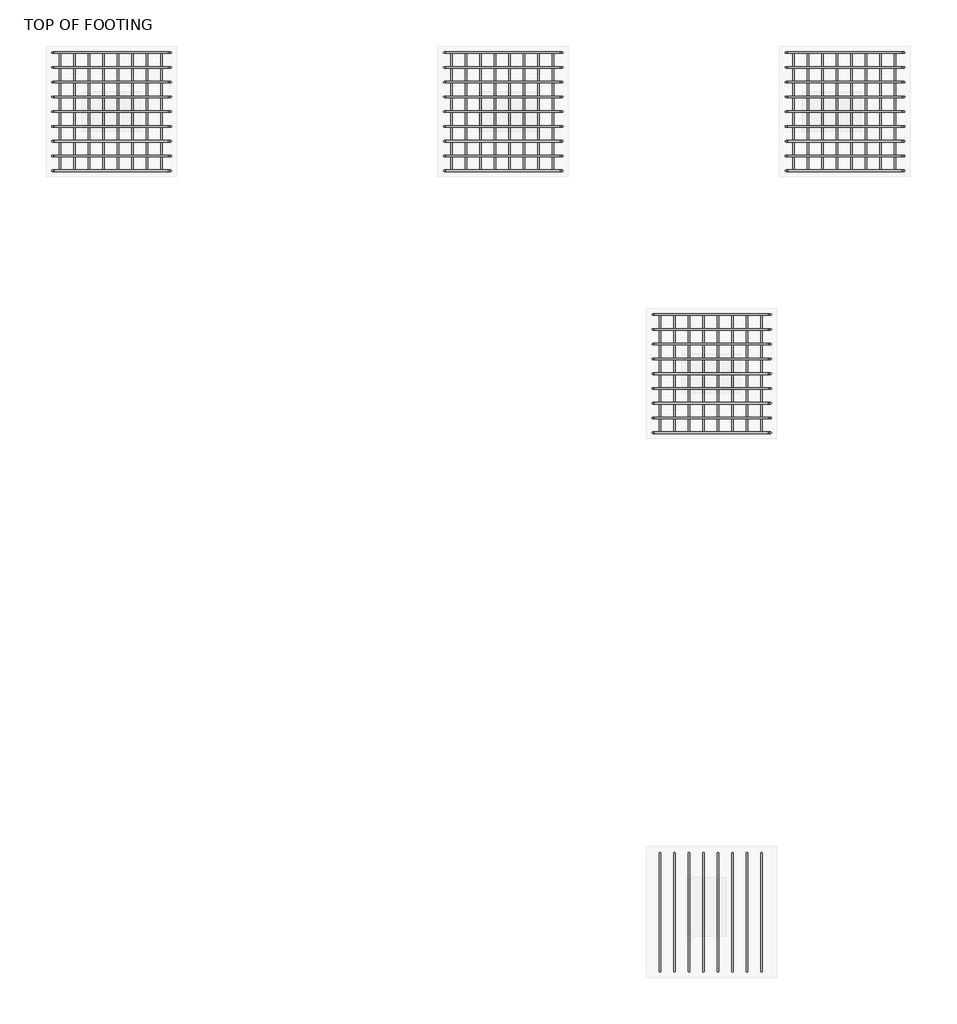
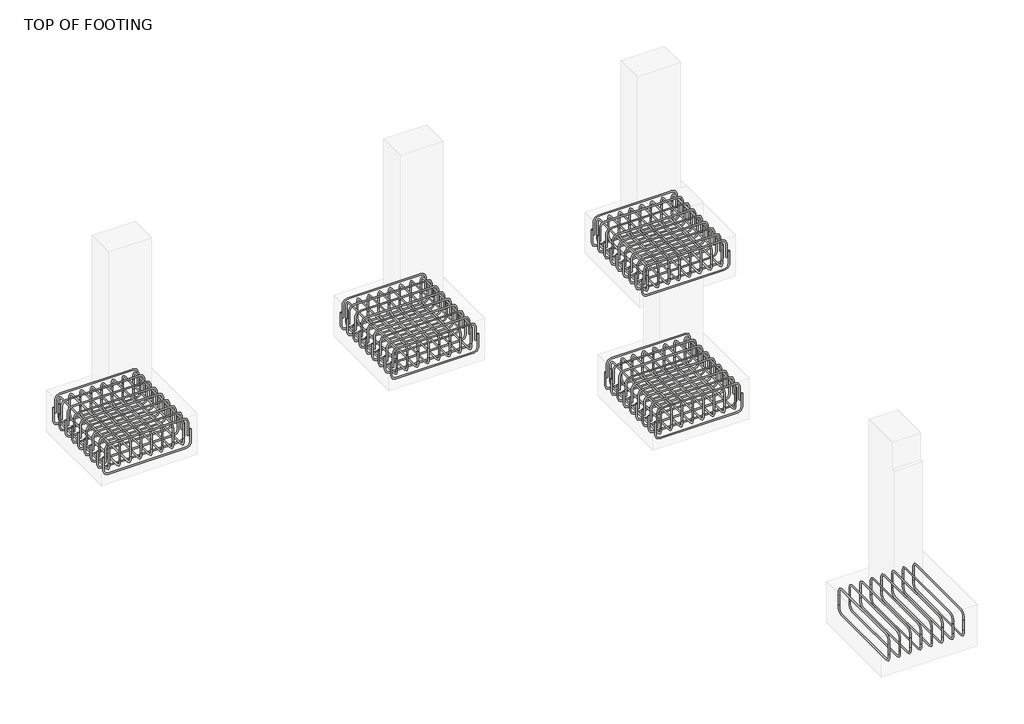
# One storey, part 14 of 20: 18 reinforcing bars.
"""IFC4 building model written with IfcOpenShell, lengths in millimetres."""

from ifc_helpers import new_model, si_unit, point, frame, origin, place, context, project, spatial, polyline, circle_curve, trimmed, segment, composite_curve, source, transform, mapped, element, save
from ifc_brep_helpers import swept_disk

model = new_model("IFC4")

# Units and contexts
model_context = context("Model", 3, world=origin())
ifc_project = project(units=[si_unit("LENGTHUNIT", "METRE", prefix="MILLI")], contexts=[model_context])

# Site, building, storey
site = spatial("IfcSite", under=ifc_project)
building = spatial("IfcBuilding", under=site)
storey = spatial("IfcBuildingStorey", under=building, Name="TOP OF FOOTING", Elevation=-1828.8)

# Reinforcing bars
placement = place(None, origin())
reinforcing_bar_shape = source(origin(), model_context, "Body", "SolidModel", [
    swept_disk(composite_curve([segment(polyline([(4636.1748054, 7703.3576276, -2006.6587682), (4636.1748054, 7703.3576276, -2153.9587682)]), True, "CONTINUOUS"), segment(trimmed(circle_curve(frame((4589.8248054, 7703.3576276, -2153.9587682), z_axis=(0.0, 1.0, 0.0), x_axis=(46.350000000000364, 0.0, 0.0)), 46.35), [point((4636.1748054, 7703.3576276, -2153.9587682))], [point((4589.8248054, 7703.3576276, -2200.3087682))], True, "CARTESIAN"), True, "CONTINUOUS"), segment(polyline([(4589.8248054, 7703.3576276, -2200.3087682), (3775.2248054, 7703.3576276, -2200.3087682)]), True, "CONTINUOUS"), segment(trimmed(circle_curve(frame((3775.2248054, 7703.3576276, -2153.9587682), z_axis=(0.0, 1.0, 0.0), x_axis=(0.0, 0.0, -46.34999999999991)), 46.35), [point((3775.2248054, 7703.3576276, -2200.3087682))], [point((3728.8748054, 7703.3576276, -2153.9587682))], True, "CARTESIAN"), True, "CONTINUOUS"), segment(polyline([(3728.8748054, 7703.3576276, -2153.9587682), (3728.8748054, 7703.3576276, -2006.6587682)]), True, "CONTINUOUS")], self_intersect=False), 6.35),
])
element("IfcReinforcingBar", 1, at=placement, inside=storey, context=model_context, shape_type="MappedRepresentation", body=[
    mapped(reinforcing_bar_shape, transform((0.0, 0.0, 0.0), x_axis=(1.0, 0.0, 0.0), y_axis=(0.0, 1.0, 0.0), z_axis=(0.0, 0.0, 1.0))),
    mapped(reinforcing_bar_shape, transform((0.0, -113.4125, 0.0), x_axis=(1.0, 0.0, 0.0), y_axis=(0.0, 1.0, 0.0), z_axis=(0.0, 0.0, 1.0))),
    mapped(reinforcing_bar_shape, transform((0.0, -226.825, 0.0), x_axis=(1.0, 0.0, 0.0), y_axis=(0.0, 1.0, 0.0), z_axis=(0.0, 0.0, 1.0))),
    mapped(reinforcing_bar_shape, transform((0.0, -340.2375, 0.0), x_axis=(1.0, 0.0, 0.0), y_axis=(0.0, 1.0, 0.0), z_axis=(0.0, 0.0, 1.0))),
    mapped(reinforcing_bar_shape, transform((0.0, -453.65, 0.0), x_axis=(1.0, 0.0, 0.0), y_axis=(0.0, 1.0, 0.0), z_axis=(0.0, 0.0, 1.0))),
    mapped(reinforcing_bar_shape, transform((0.0, -567.0625, 0.0), x_axis=(1.0, 0.0, 0.0), y_axis=(0.0, 1.0, 0.0), z_axis=(0.0, 0.0, 1.0))),
    mapped(reinforcing_bar_shape, transform((0.0, -680.475, 0.0), x_axis=(1.0, 0.0, 0.0), y_axis=(0.0, 1.0, 0.0), z_axis=(0.0, 0.0, 1.0))),
    mapped(reinforcing_bar_shape, transform((0.0, -793.8875, 0.0), x_axis=(1.0, 0.0, 0.0), y_axis=(0.0, 1.0, 0.0), z_axis=(0.0, 0.0, 1.0))),
    mapped(reinforcing_bar_shape, transform((0.0, -907.3, 0.0), x_axis=(1.0, 0.0, 0.0), y_axis=(0.0, 1.0, 0.0), z_axis=(0.0, 0.0, 1.0))),
])
reinforcing_bar_2_shape = source(origin(), model_context, "Body", "SolidModel", [
    swept_disk(composite_curve([segment(polyline([(3748.3489167, 7703.3576276, -2068.8), (3748.3489167, 7703.3576276, -1921.5)]), True, "CONTINUOUS"), segment(trimmed(circle_curve(frame((3794.6989167, 7703.3576276, -1921.5), z_axis=(0.0, 1.0, 0.0), x_axis=(-46.350000000000364, 0.0, 0.0)), 46.35), [point((3748.3489167, 7703.3576276, -1921.5))], [point((3794.6989167, 7703.3576276, -1875.15))], True, "CARTESIAN"), True, "CONTINUOUS"), segment(polyline([(3794.6989167, 7703.3576276, -1875.15), (4564.1623164, 7703.3576276, -1875.15)]), True, "CONTINUOUS"), segment(trimmed(circle_curve(frame((4564.1623164, 7703.3576276, -1921.5), z_axis=(0.0, 1.0, 0.0), x_axis=(0.0, 0.0, 46.34999999999991)), 46.35), [point((4564.1623164, 7703.3576276, -1875.15))], [point((4610.5123164, 7703.3576276, -1921.5))], True, "CARTESIAN"), True, "CONTINUOUS"), segment(polyline([(4610.5123164, 7703.3576276, -1921.5), (4610.5123164, 7703.3576276, -2068.8)]), True, "CONTINUOUS")], self_intersect=False), 6.35),
])
element("IfcReinforcingBar", 2, at=placement, inside=storey, context=model_context, shape_type="MappedRepresentation", body=[
    mapped(reinforcing_bar_2_shape, transform((0.0, 0.0, 0.0), x_axis=(1.0, 0.0, 0.0), y_axis=(0.0, 1.0, 0.0), z_axis=(0.0, 0.0, 1.0))),
    mapped(reinforcing_bar_2_shape, transform((0.0, -113.4125, 0.0), x_axis=(1.0, 0.0, 0.0), y_axis=(0.0, 1.0, 0.0), z_axis=(0.0, 0.0, 1.0))),
    mapped(reinforcing_bar_2_shape, transform((0.0, -226.825, 0.0), x_axis=(1.0, 0.0, 0.0), y_axis=(0.0, 1.0, 0.0), z_axis=(0.0, 0.0, 1.0))),
    mapped(reinforcing_bar_2_shape, transform((0.0, -340.2375, 0.0), x_axis=(1.0, 0.0, 0.0), y_axis=(0.0, 1.0, 0.0), z_axis=(0.0, 0.0, 1.0))),
    mapped(reinforcing_bar_2_shape, transform((0.0, -453.65, 0.0), x_axis=(1.0, 0.0, 0.0), y_axis=(0.0, 1.0, 0.0), z_axis=(0.0, 0.0, 1.0))),
    mapped(reinforcing_bar_2_shape, transform((0.0, -567.0625, 0.0), x_axis=(1.0, 0.0, 0.0), y_axis=(0.0, 1.0, 0.0), z_axis=(0.0, 0.0, 1.0))),
    mapped(reinforcing_bar_2_shape, transform((0.0, -680.475, 0.0), x_axis=(1.0, 0.0, 0.0), y_axis=(0.0, 1.0, 0.0), z_axis=(0.0, 0.0, 1.0))),
    mapped(reinforcing_bar_2_shape, transform((0.0, -793.8875, 0.0), x_axis=(1.0, 0.0, 0.0), y_axis=(0.0, 1.0, 0.0), z_axis=(0.0, 0.0, 1.0))),
    mapped(reinforcing_bar_2_shape, transform((0.0, -907.3, 0.0), x_axis=(1.0, 0.0, 0.0), y_axis=(0.0, 1.0, 0.0), z_axis=(0.0, 0.0, 1.0))),
])
reinforcing_bar_3_shape = source(origin(), model_context, "Body", "SolidModel", [
    swept_disk(composite_curve([segment(polyline([(4564.677844, 7703.3576276, -2086.1951968), (4564.677844, 7703.3576276, -1938.8951968)]), True, "CONTINUOUS"), segment(trimmed(circle_curve(frame((4564.677844, 7657.0076276, -1938.8951968), z_axis=(1.0, 0.0, 0.0), x_axis=(0.0, 46.350000000000364, 0.0)), 46.35), [point((4564.677844, 7703.3576276, -1938.8951968))], [point((4564.677844, 7657.0076276, -1892.5451968))], True, "CARTESIAN"), True, "CONTINUOUS"), segment(polyline([(4564.677844, 7657.0076276, -1892.5451968), (4564.677844, 6842.4076276, -1892.5451968)]), True, "CONTINUOUS"), segment(trimmed(circle_curve(frame((4564.677844, 6842.4076276, -1938.8951968), z_axis=(1.0, 0.0, 0.0), x_axis=(0.0, 0.0, 46.34999999999991)), 46.35), [point((4564.677844, 6842.4076276, -1892.5451968))], [point((4564.677844, 6796.0576276, -1938.8951968))], True, "CARTESIAN"), True, "CONTINUOUS"), segment(polyline([(4564.677844, 6796.0576276, -1938.8951968), (4564.677844, 6796.0576276, -2086.1951968)]), True, "CONTINUOUS")], self_intersect=False), 6.35),
])
element("IfcReinforcingBar", 3, at=placement, inside=storey, context=model_context, shape_type="MappedRepresentation", body=[
    mapped(reinforcing_bar_3_shape, transform((0.0, 0.0, 0.0), x_axis=(1.0, 0.0, 0.0), y_axis=(0.0, 1.0, 0.0), z_axis=(0.0, 0.0, 1.0))),
    mapped(reinforcing_bar_3_shape, transform((-111.2862402, 0.0, 0.0), x_axis=(1.0, 0.0, 0.0), y_axis=(0.0, 1.0, 0.0), z_axis=(0.0, 0.0, 1.0))),
    mapped(reinforcing_bar_3_shape, transform((-222.5724804, 0.0, 0.0), x_axis=(1.0, 0.0, 0.0), y_axis=(0.0, 1.0, 0.0), z_axis=(0.0, 0.0, 1.0))),
    mapped(reinforcing_bar_3_shape, transform((-333.8587205, 0.0, 0.0), x_axis=(1.0, 0.0, 0.0), y_axis=(0.0, 1.0, 0.0), z_axis=(0.0, 0.0, 1.0))),
    mapped(reinforcing_bar_3_shape, transform((-445.1449607, 0.0, 0.0), x_axis=(1.0, 0.0, 0.0), y_axis=(0.0, 1.0, 0.0), z_axis=(0.0, 0.0, 1.0))),
    mapped(reinforcing_bar_3_shape, transform((-556.4312009, 0.0, 0.0), x_axis=(1.0, 0.0, 0.0), y_axis=(0.0, 1.0, 0.0), z_axis=(0.0, 0.0, 1.0))),
    mapped(reinforcing_bar_3_shape, transform((-667.7174411, 0.0, 0.0), x_axis=(1.0, 0.0, 0.0), y_axis=(0.0, 1.0, 0.0), z_axis=(0.0, 0.0, 1.0))),
    mapped(reinforcing_bar_3_shape, transform((-779.0036813, 0.0, 0.0), x_axis=(1.0, 0.0, 0.0), y_axis=(0.0, 1.0, 0.0), z_axis=(0.0, 0.0, 1.0))),
])
reinforcing_bar_4_shape = source(origin(), model_context, "Body", "SolidModel", [
    swept_disk(composite_curve([segment(polyline([(3785.6741627, 7703.3576276, -1979.1645013), (3785.6741627, 7703.3576276, -2126.4645013)]), True, "CONTINUOUS"), segment(trimmed(circle_curve(frame((3785.6741627, 7657.0076276, -2126.4645013), z_axis=(-1.0, 0.0, 0.0), x_axis=(0.0, 46.350000000000364, 0.0)), 46.35), [point((3785.6741627, 7703.3576276, -2126.4645013))], [point((3785.6741627, 7657.0076276, -2172.8145013))], True, "CARTESIAN"), True, "CONTINUOUS"), segment(polyline([(3785.6741627, 7657.0076276, -2172.8145013), (3785.6741627, 6842.4076276, -2172.8145013)]), True, "CONTINUOUS"), segment(trimmed(circle_curve(frame((3785.6741627, 6842.4076276, -2126.4645013), z_axis=(-1.0, 0.0, 0.0), x_axis=(0.0, 0.0, -46.34999999999991)), 46.35), [point((3785.6741627, 6842.4076276, -2172.8145013))], [point((3785.6741627, 6796.0576276, -2126.4645013))], True, "CARTESIAN"), True, "CONTINUOUS"), segment(polyline([(3785.6741627, 6796.0576276, -2126.4645013), (3785.6741627, 6796.0576276, -1979.1645013)]), True, "CONTINUOUS")], self_intersect=False), 6.35),
])
element("IfcReinforcingBar", 4, at=placement, inside=storey, context=model_context, shape_type="MappedRepresentation", body=[
    mapped(reinforcing_bar_4_shape, transform((0.0, 0.0, 0.0), x_axis=(1.0, 0.0, 0.0), y_axis=(0.0, 1.0, 0.0), z_axis=(0.0, 0.0, 1.0))),
    mapped(reinforcing_bar_4_shape, transform((111.2862402, 0.0, 0.0), x_axis=(1.0, 0.0, 0.0), y_axis=(0.0, 1.0, 0.0), z_axis=(0.0, 0.0, 1.0))),
    mapped(reinforcing_bar_4_shape, transform((222.5724804, 0.0, 0.0), x_axis=(1.0, 0.0, 0.0), y_axis=(0.0, 1.0, 0.0), z_axis=(0.0, 0.0, 1.0))),
    mapped(reinforcing_bar_4_shape, transform((333.8587205, 0.0, 0.0), x_axis=(1.0, 0.0, 0.0), y_axis=(0.0, 1.0, 0.0), z_axis=(0.0, 0.0, 1.0))),
    mapped(reinforcing_bar_4_shape, transform((445.1449607, 0.0, 0.0), x_axis=(1.0, 0.0, 0.0), y_axis=(0.0, 1.0, 0.0), z_axis=(0.0, 0.0, 1.0))),
    mapped(reinforcing_bar_4_shape, transform((556.4312009, 0.0, 0.0), x_axis=(1.0, 0.0, 0.0), y_axis=(0.0, 1.0, 0.0), z_axis=(0.0, 0.0, 1.0))),
    mapped(reinforcing_bar_4_shape, transform((667.7174411, 0.0, 0.0), x_axis=(1.0, 0.0, 0.0), y_axis=(0.0, 1.0, 0.0), z_axis=(0.0, 0.0, 1.0))),
    mapped(reinforcing_bar_4_shape, transform((779.0036813, 0.0, 0.0), x_axis=(1.0, 0.0, 0.0), y_axis=(0.0, 1.0, 0.0), z_axis=(0.0, 0.0, 1.0))),
])
reinforcing_bar_5_shape = source(origin(), model_context, "Body", "SolidModel", [
    swept_disk(composite_curve([segment(polyline([(7260.5179014, 7703.3576276, -2006.6587682), (7260.5179014, 7703.3576276, -2153.9587682)]), True, "CONTINUOUS"), segment(trimmed(circle_curve(frame((7214.1679014, 7703.3576276, -2153.9587682), z_axis=(0.0, 1.0, 0.0), x_axis=(46.349999999999454, 0.0, 0.0)), 46.35), [point((7260.5179014, 7703.3576276, -2153.9587682))], [point((7214.1679014, 7703.3576276, -2200.3087682))], True, "CARTESIAN"), True, "CONTINUOUS"), segment(polyline([(7214.1679014, 7703.3576276, -2200.3087682), (6399.5679014, 7703.3576276, -2200.3087682)]), True, "CONTINUOUS"), segment(trimmed(circle_curve(frame((6399.5679014, 7703.3576276, -2153.9587682), z_axis=(0.0, 1.0, 0.0), x_axis=(0.0, 0.0, -46.34999999999991)), 46.35), [point((6399.5679014, 7703.3576276, -2200.3087682))], [point((6353.2179014, 7703.3576276, -2153.9587682))], True, "CARTESIAN"), True, "CONTINUOUS"), segment(polyline([(6353.2179014, 7703.3576276, -2153.9587682), (6353.2179014, 7703.3576276, -2006.6587682)]), True, "CONTINUOUS")], self_intersect=False), 6.35),
])
element("IfcReinforcingBar", 5, at=placement, inside=storey, context=model_context, shape_type="MappedRepresentation", body=[
    mapped(reinforcing_bar_5_shape, transform((0.0, 0.0, 0.0), x_axis=(1.0, 0.0, 0.0), y_axis=(0.0, 1.0, 0.0), z_axis=(0.0, 0.0, 1.0))),
    mapped(reinforcing_bar_5_shape, transform((0.0, -113.4125, 0.0), x_axis=(1.0, 0.0, 0.0), y_axis=(0.0, 1.0, 0.0), z_axis=(0.0, 0.0, 1.0))),
    mapped(reinforcing_bar_5_shape, transform((0.0, -226.825, 0.0), x_axis=(1.0, 0.0, 0.0), y_axis=(0.0, 1.0, 0.0), z_axis=(0.0, 0.0, 1.0))),
    mapped(reinforcing_bar_5_shape, transform((0.0, -340.2375, 0.0), x_axis=(1.0, 0.0, 0.0), y_axis=(0.0, 1.0, 0.0), z_axis=(0.0, 0.0, 1.0))),
    mapped(reinforcing_bar_5_shape, transform((0.0, -453.65, 0.0), x_axis=(1.0, 0.0, 0.0), y_axis=(0.0, 1.0, 0.0), z_axis=(0.0, 0.0, 1.0))),
    mapped(reinforcing_bar_5_shape, transform((0.0, -567.0625, 0.0), x_axis=(1.0, 0.0, 0.0), y_axis=(0.0, 1.0, 0.0), z_axis=(0.0, 0.0, 1.0))),
    mapped(reinforcing_bar_5_shape, transform((0.0, -680.475, 0.0), x_axis=(1.0, 0.0, 0.0), y_axis=(0.0, 1.0, 0.0), z_axis=(0.0, 0.0, 1.0))),
    mapped(reinforcing_bar_5_shape, transform((0.0, -793.8875, 0.0), x_axis=(1.0, 0.0, 0.0), y_axis=(0.0, 1.0, 0.0), z_axis=(0.0, 0.0, 1.0))),
    mapped(reinforcing_bar_5_shape, transform((0.0, -907.3, 0.0), x_axis=(1.0, 0.0, 0.0), y_axis=(0.0, 1.0, 0.0), z_axis=(0.0, 0.0, 1.0))),
])
reinforcing_bar_6_shape = source(origin(), model_context, "Body", "SolidModel", [
    swept_disk(composite_curve([segment(polyline([(6372.6920127, 7703.3576276, -2068.8), (6372.6920127, 7703.3576276, -1921.5)]), True, "CONTINUOUS"), segment(trimmed(circle_curve(frame((6419.0420127, 7703.3576276, -1921.5), z_axis=(0.0, 1.0, 0.0), x_axis=(-46.349999999999454, 0.0, 0.0)), 46.35), [point((6372.6920127, 7703.3576276, -1921.5))], [point((6419.0420127, 7703.3576276, -1875.15))], True, "CARTESIAN"), True, "CONTINUOUS"), segment(polyline([(6419.0420127, 7703.3576276, -1875.15), (7188.5054124, 7703.3576276, -1875.15)]), True, "CONTINUOUS"), segment(trimmed(circle_curve(frame((7188.5054124, 7703.3576276, -1921.5), z_axis=(0.0, 1.0, 0.0), x_axis=(0.0, 0.0, 46.34999999999991)), 46.35), [point((7188.5054124, 7703.3576276, -1875.15))], [point((7234.8554124, 7703.3576276, -1921.5))], True, "CARTESIAN"), True, "CONTINUOUS"), segment(polyline([(7234.8554124, 7703.3576276, -1921.5), (7234.8554124, 7703.3576276, -2068.8)]), True, "CONTINUOUS")], self_intersect=False), 6.35),
])
element("IfcReinforcingBar", 6, at=placement, inside=storey, context=model_context, shape_type="MappedRepresentation", body=[
    mapped(reinforcing_bar_6_shape, transform((0.0, 0.0, 0.0), x_axis=(1.0, 0.0, 0.0), y_axis=(0.0, 1.0, 0.0), z_axis=(0.0, 0.0, 1.0))),
    mapped(reinforcing_bar_6_shape, transform((0.0, -113.4125, 0.0), x_axis=(1.0, 0.0, 0.0), y_axis=(0.0, 1.0, 0.0), z_axis=(0.0, 0.0, 1.0))),
    mapped(reinforcing_bar_6_shape, transform((0.0, -226.825, 0.0), x_axis=(1.0, 0.0, 0.0), y_axis=(0.0, 1.0, 0.0), z_axis=(0.0, 0.0, 1.0))),
    mapped(reinforcing_bar_6_shape, transform((0.0, -340.2375, 0.0), x_axis=(1.0, 0.0, 0.0), y_axis=(0.0, 1.0, 0.0), z_axis=(0.0, 0.0, 1.0))),
    mapped(reinforcing_bar_6_shape, transform((0.0, -453.65, 0.0), x_axis=(1.0, 0.0, 0.0), y_axis=(0.0, 1.0, 0.0), z_axis=(0.0, 0.0, 1.0))),
    mapped(reinforcing_bar_6_shape, transform((0.0, -567.0625, 0.0), x_axis=(1.0, 0.0, 0.0), y_axis=(0.0, 1.0, 0.0), z_axis=(0.0, 0.0, 1.0))),
    mapped(reinforcing_bar_6_shape, transform((0.0, -680.475, 0.0), x_axis=(1.0, 0.0, 0.0), y_axis=(0.0, 1.0, 0.0), z_axis=(0.0, 0.0, 1.0))),
    mapped(reinforcing_bar_6_shape, transform((0.0, -793.8875, 0.0), x_axis=(1.0, 0.0, 0.0), y_axis=(0.0, 1.0, 0.0), z_axis=(0.0, 0.0, 1.0))),
    mapped(reinforcing_bar_6_shape, transform((0.0, -907.3, 0.0), x_axis=(1.0, 0.0, 0.0), y_axis=(0.0, 1.0, 0.0), z_axis=(0.0, 0.0, 1.0))),
])
reinforcing_bar_7_shape = source(origin(), model_context, "Body", "SolidModel", [
    swept_disk(composite_curve([segment(polyline([(7189.02094, 7703.3576276, -2086.1951968), (7189.02094, 7703.3576276, -1938.8951968)]), True, "CONTINUOUS"), segment(trimmed(circle_curve(frame((7189.02094, 7657.0076276, -1938.8951968), z_axis=(1.0, 0.0, 0.0), x_axis=(0.0, 46.350000000000364, 0.0)), 46.35), [point((7189.02094, 7703.3576276, -1938.8951968))], [point((7189.02094, 7657.0076276, -1892.5451968))], True, "CARTESIAN"), True, "CONTINUOUS"), segment(polyline([(7189.02094, 7657.0076276, -1892.5451968), (7189.02094, 6842.4076276, -1892.5451968)]), True, "CONTINUOUS"), segment(trimmed(circle_curve(frame((7189.02094, 6842.4076276, -1938.8951968), z_axis=(1.0, 0.0, 0.0), x_axis=(0.0, 0.0, 46.34999999999991)), 46.35), [point((7189.02094, 6842.4076276, -1892.5451968))], [point((7189.02094, 6796.0576276, -1938.8951968))], True, "CARTESIAN"), True, "CONTINUOUS"), segment(polyline([(7189.02094, 6796.0576276, -1938.8951968), (7189.02094, 6796.0576276, -2086.1951968)]), True, "CONTINUOUS")], self_intersect=False), 6.35),
])
element("IfcReinforcingBar", 7, at=placement, inside=storey, context=model_context, shape_type="MappedRepresentation", body=[
    mapped(reinforcing_bar_7_shape, transform((0.0, 0.0, 0.0), x_axis=(1.0, 0.0, 0.0), y_axis=(0.0, 1.0, 0.0), z_axis=(0.0, 0.0, 1.0))),
    mapped(reinforcing_bar_7_shape, transform((-111.2862402, 0.0, 0.0), x_axis=(1.0, 0.0, 0.0), y_axis=(0.0, 1.0, 0.0), z_axis=(0.0, 0.0, 1.0))),
    mapped(reinforcing_bar_7_shape, transform((-222.5724804, 0.0, 0.0), x_axis=(1.0, 0.0, 0.0), y_axis=(0.0, 1.0, 0.0), z_axis=(0.0, 0.0, 1.0))),
    mapped(reinforcing_bar_7_shape, transform((-333.8587205, 0.0, 0.0), x_axis=(1.0, 0.0, 0.0), y_axis=(0.0, 1.0, 0.0), z_axis=(0.0, 0.0, 1.0))),
    mapped(reinforcing_bar_7_shape, transform((-445.1449607, 0.0, 0.0), x_axis=(1.0, 0.0, 0.0), y_axis=(0.0, 1.0, 0.0), z_axis=(0.0, 0.0, 1.0))),
    mapped(reinforcing_bar_7_shape, transform((-556.4312009, 0.0, 0.0), x_axis=(1.0, 0.0, 0.0), y_axis=(0.0, 1.0, 0.0), z_axis=(0.0, 0.0, 1.0))),
    mapped(reinforcing_bar_7_shape, transform((-667.7174411, 0.0, 0.0), x_axis=(1.0, 0.0, 0.0), y_axis=(0.0, 1.0, 0.0), z_axis=(0.0, 0.0, 1.0))),
    mapped(reinforcing_bar_7_shape, transform((-779.0036813, 0.0, 0.0), x_axis=(1.0, 0.0, 0.0), y_axis=(0.0, 1.0, 0.0), z_axis=(0.0, 0.0, 1.0))),
])
reinforcing_bar_8_shape = source(origin(), model_context, "Body", "SolidModel", [
    swept_disk(composite_curve([segment(polyline([(6410.0172587, 7703.3576276, -1979.1645013), (6410.0172587, 7703.3576276, -2126.4645013)]), True, "CONTINUOUS"), segment(trimmed(circle_curve(frame((6410.0172587, 7657.0076276, -2126.4645013), z_axis=(-1.0, 0.0, 0.0), x_axis=(0.0, 46.350000000000364, 0.0)), 46.35), [point((6410.0172587, 7703.3576276, -2126.4645013))], [point((6410.0172587, 7657.0076276, -2172.8145013))], True, "CARTESIAN"), True, "CONTINUOUS"), segment(polyline([(6410.0172587, 7657.0076276, -2172.8145013), (6410.0172587, 6842.4076276, -2172.8145013)]), True, "CONTINUOUS"), segment(trimmed(circle_curve(frame((6410.0172587, 6842.4076276, -2126.4645013), z_axis=(-1.0, 0.0, 0.0), x_axis=(0.0, 0.0, -46.34999999999991)), 46.35), [point((6410.0172587, 6842.4076276, -2172.8145013))], [point((6410.0172587, 6796.0576276, -2126.4645013))], True, "CARTESIAN"), True, "CONTINUOUS"), segment(polyline([(6410.0172587, 6796.0576276, -2126.4645013), (6410.0172587, 6796.0576276, -1979.1645013)]), True, "CONTINUOUS")], self_intersect=False), 6.35),
])
element("IfcReinforcingBar", 8, at=placement, inside=storey, context=model_context, shape_type="MappedRepresentation", body=[
    mapped(reinforcing_bar_8_shape, transform((0.0, 0.0, 0.0), x_axis=(1.0, 0.0, 0.0), y_axis=(0.0, 1.0, 0.0), z_axis=(0.0, 0.0, 1.0))),
    mapped(reinforcing_bar_8_shape, transform((111.2862402, 0.0, 0.0), x_axis=(1.0, 0.0, 0.0), y_axis=(0.0, 1.0, 0.0), z_axis=(0.0, 0.0, 1.0))),
    mapped(reinforcing_bar_8_shape, transform((222.5724804, 0.0, 0.0), x_axis=(1.0, 0.0, 0.0), y_axis=(0.0, 1.0, 0.0), z_axis=(0.0, 0.0, 1.0))),
    mapped(reinforcing_bar_8_shape, transform((333.8587205, 0.0, 0.0), x_axis=(1.0, 0.0, 0.0), y_axis=(0.0, 1.0, 0.0), z_axis=(0.0, 0.0, 1.0))),
    mapped(reinforcing_bar_8_shape, transform((445.1449607, 0.0, 0.0), x_axis=(1.0, 0.0, 0.0), y_axis=(0.0, 1.0, 0.0), z_axis=(0.0, 0.0, 1.0))),
    mapped(reinforcing_bar_8_shape, transform((556.4312009, 0.0, 0.0), x_axis=(1.0, 0.0, 0.0), y_axis=(0.0, 1.0, 0.0), z_axis=(0.0, 0.0, 1.0))),
    mapped(reinforcing_bar_8_shape, transform((667.7174411, 0.0, 0.0), x_axis=(1.0, 0.0, 0.0), y_axis=(0.0, 1.0, 0.0), z_axis=(0.0, 0.0, 1.0))),
    mapped(reinforcing_bar_8_shape, transform((779.0036813, 0.0, 0.0), x_axis=(1.0, 0.0, 0.0), y_axis=(0.0, 1.0, 0.0), z_axis=(0.0, 0.0, 1.0))),
])
reinforcing_bar_9_shape = source(origin(), model_context, "Body", "SolidModel", [
    swept_disk(composite_curve([segment(polyline([(6164.677844, 1554.8213929, -2086.1951968), (6164.677844, 1554.8213929, -1938.8951968)]), True, "CONTINUOUS"), segment(trimmed(circle_curve(frame((6164.677844, 1508.4713929, -1938.8951968), z_axis=(1.0, 0.0, 0.0), x_axis=(0.0, 46.350000000000136, 0.0)), 46.35), [point((6164.677844, 1554.8213929, -1938.8951968))], [point((6164.677844, 1508.4713929, -1892.5451968))], True, "CARTESIAN"), True, "CONTINUOUS"), segment(polyline([(6164.677844, 1508.4713929, -1892.5451968), (6164.677844, 693.8713929, -1892.5451968)]), True, "CONTINUOUS"), segment(trimmed(circle_curve(frame((6164.677844, 693.8713929, -1938.8951968), z_axis=(1.0, 0.0, 0.0), x_axis=(0.0, 0.0, 46.34999999999991)), 46.35), [point((6164.677844, 693.8713929, -1892.5451968))], [point((6164.677844, 647.5213929, -1938.8951968))], True, "CARTESIAN"), True, "CONTINUOUS"), segment(polyline([(6164.677844, 647.5213929, -1938.8951968), (6164.677844, 647.5213929, -2086.1951968)]), True, "CONTINUOUS")], self_intersect=False), 6.35),
])
element("IfcReinforcingBar", 9, at=placement, inside=storey, context=model_context, shape_type="MappedRepresentation", body=[
    mapped(reinforcing_bar_9_shape, transform((0.0, 0.0, 0.0), x_axis=(1.0, 0.0, 0.0), y_axis=(0.0, 1.0, 0.0), z_axis=(0.0, 0.0, 1.0))),
    mapped(reinforcing_bar_9_shape, transform((-111.2862402, 0.0, 0.0), x_axis=(1.0, 0.0, 0.0), y_axis=(0.0, 1.0, 0.0), z_axis=(0.0, 0.0, 1.0))),
    mapped(reinforcing_bar_9_shape, transform((-222.5724804, 0.0, 0.0), x_axis=(1.0, 0.0, 0.0), y_axis=(0.0, 1.0, 0.0), z_axis=(0.0, 0.0, 1.0))),
    mapped(reinforcing_bar_9_shape, transform((-333.8587205, 0.0, 0.0), x_axis=(1.0, 0.0, 0.0), y_axis=(0.0, 1.0, 0.0), z_axis=(0.0, 0.0, 1.0))),
    mapped(reinforcing_bar_9_shape, transform((-445.1449607, 0.0, 0.0), x_axis=(1.0, 0.0, 0.0), y_axis=(0.0, 1.0, 0.0), z_axis=(0.0, 0.0, 1.0))),
    mapped(reinforcing_bar_9_shape, transform((-556.4312009, 0.0, 0.0), x_axis=(1.0, 0.0, 0.0), y_axis=(0.0, 1.0, 0.0), z_axis=(0.0, 0.0, 1.0))),
    mapped(reinforcing_bar_9_shape, transform((-667.7174411, 0.0, 0.0), x_axis=(1.0, 0.0, 0.0), y_axis=(0.0, 1.0, 0.0), z_axis=(0.0, 0.0, 1.0))),
    mapped(reinforcing_bar_9_shape, transform((-779.0036813, 0.0, 0.0), x_axis=(1.0, 0.0, 0.0), y_axis=(0.0, 1.0, 0.0), z_axis=(0.0, 0.0, 1.0))),
])
reinforcing_bar_10_shape = source(origin(), model_context, "Body", "SolidModel", [
    swept_disk(composite_curve([segment(polyline([(5385.6741627, 1554.8213929, -1979.1645013), (5385.6741627, 1554.8213929, -2126.4645013)]), True, "CONTINUOUS"), segment(trimmed(circle_curve(frame((5385.6741627, 1508.4713929, -2126.4645013), z_axis=(-1.0, 0.0, 0.0), x_axis=(0.0, 46.350000000000136, 0.0)), 46.35), [point((5385.6741627, 1554.8213929, -2126.4645013))], [point((5385.6741627, 1508.4713929, -2172.8145013))], True, "CARTESIAN"), True, "CONTINUOUS"), segment(polyline([(5385.6741627, 1508.4713929, -2172.8145013), (5385.6741627, 693.8713929, -2172.8145013)]), True, "CONTINUOUS"), segment(trimmed(circle_curve(frame((5385.6741627, 693.8713929, -2126.4645013), z_axis=(-1.0, 0.0, 0.0), x_axis=(0.0, 0.0, -46.34999999999991)), 46.35), [point((5385.6741627, 693.8713929, -2172.8145013))], [point((5385.6741627, 647.5213929, -2126.4645013))], True, "CARTESIAN"), True, "CONTINUOUS"), segment(polyline([(5385.6741627, 647.5213929, -2126.4645013), (5385.6741627, 647.5213929, -1979.1645013)]), True, "CONTINUOUS")], self_intersect=False), 6.35),
])
element("IfcReinforcingBar", 10, at=placement, inside=storey, context=model_context, shape_type="MappedRepresentation", body=[
    mapped(reinforcing_bar_10_shape, transform((0.0, 0.0, 0.0), x_axis=(1.0, 0.0, 0.0), y_axis=(0.0, 1.0, 0.0), z_axis=(0.0, 0.0, 1.0))),
    mapped(reinforcing_bar_10_shape, transform((111.2862402, 0.0, 0.0), x_axis=(1.0, 0.0, 0.0), y_axis=(0.0, 1.0, 0.0), z_axis=(0.0, 0.0, 1.0))),
    mapped(reinforcing_bar_10_shape, transform((222.5724804, 0.0, 0.0), x_axis=(1.0, 0.0, 0.0), y_axis=(0.0, 1.0, 0.0), z_axis=(0.0, 0.0, 1.0))),
    mapped(reinforcing_bar_10_shape, transform((333.8587205, 0.0, 0.0), x_axis=(1.0, 0.0, 0.0), y_axis=(0.0, 1.0, 0.0), z_axis=(0.0, 0.0, 1.0))),
    mapped(reinforcing_bar_10_shape, transform((445.1449607, 0.0, 0.0), x_axis=(1.0, 0.0, 0.0), y_axis=(0.0, 1.0, 0.0), z_axis=(0.0, 0.0, 1.0))),
    mapped(reinforcing_bar_10_shape, transform((556.4312009, 0.0, 0.0), x_axis=(1.0, 0.0, 0.0), y_axis=(0.0, 1.0, 0.0), z_axis=(0.0, 0.0, 1.0))),
    mapped(reinforcing_bar_10_shape, transform((667.7174411, 0.0, 0.0), x_axis=(1.0, 0.0, 0.0), y_axis=(0.0, 1.0, 0.0), z_axis=(0.0, 0.0, 1.0))),
    mapped(reinforcing_bar_10_shape, transform((779.0036813, 0.0, 0.0), x_axis=(1.0, 0.0, 0.0), y_axis=(0.0, 1.0, 0.0), z_axis=(0.0, 0.0, 1.0))),
])
reinforcing_bar_11_shape = source(origin(), model_context, "Body", "SolidModel", [
    swept_disk(composite_curve([segment(polyline([(1628.3796816, 7703.3576276, -2006.6587682), (1628.3796816, 7703.3576276, -2153.9587682)]), True, "CONTINUOUS"), segment(trimmed(circle_curve(frame((1582.0296816, 7703.3576276, -2153.9587682), z_axis=(0.0, 1.0, 0.0), x_axis=(46.34999999999991, 0.0, 0.0)), 46.35), [point((1628.3796816, 7703.3576276, -2153.9587682))], [point((1582.0296816, 7703.3576276, -2200.3087682))], True, "CARTESIAN"), True, "CONTINUOUS"), segment(polyline([(1582.0296816, 7703.3576276, -2200.3087682), (767.4296816, 7703.3576276, -2200.3087682)]), True, "CONTINUOUS"), segment(trimmed(circle_curve(frame((767.4296816, 7703.3576276, -2153.9587682), z_axis=(0.0, 1.0, 0.0), x_axis=(0.0, 0.0, -46.34999999999991)), 46.35), [point((767.4296816, 7703.3576276, -2200.3087682))], [point((721.0796816, 7703.3576276, -2153.9587682))], True, "CARTESIAN"), True, "CONTINUOUS"), segment(polyline([(721.0796816, 7703.3576276, -2153.9587682), (721.0796816, 7703.3576276, -2006.6587682)]), True, "CONTINUOUS")], self_intersect=False), 6.35),
])
element("IfcReinforcingBar", 11, at=placement, inside=storey, context=model_context, shape_type="MappedRepresentation", body=[
    mapped(reinforcing_bar_11_shape, transform((0.0, 0.0, 0.0), x_axis=(1.0, 0.0, 0.0), y_axis=(0.0, 1.0, 0.0), z_axis=(0.0, 0.0, 1.0))),
    mapped(reinforcing_bar_11_shape, transform((0.0, -113.4125, 0.0), x_axis=(1.0, 0.0, 0.0), y_axis=(0.0, 1.0, 0.0), z_axis=(0.0, 0.0, 1.0))),
    mapped(reinforcing_bar_11_shape, transform((0.0, -226.825, 0.0), x_axis=(1.0, 0.0, 0.0), y_axis=(0.0, 1.0, 0.0), z_axis=(0.0, 0.0, 1.0))),
    mapped(reinforcing_bar_11_shape, transform((0.0, -340.2375, 0.0), x_axis=(1.0, 0.0, 0.0), y_axis=(0.0, 1.0, 0.0), z_axis=(0.0, 0.0, 1.0))),
    mapped(reinforcing_bar_11_shape, transform((0.0, -453.65, 0.0), x_axis=(1.0, 0.0, 0.0), y_axis=(0.0, 1.0, 0.0), z_axis=(0.0, 0.0, 1.0))),
    mapped(reinforcing_bar_11_shape, transform((0.0, -567.0625, 0.0), x_axis=(1.0, 0.0, 0.0), y_axis=(0.0, 1.0, 0.0), z_axis=(0.0, 0.0, 1.0))),
    mapped(reinforcing_bar_11_shape, transform((0.0, -680.475, 0.0), x_axis=(1.0, 0.0, 0.0), y_axis=(0.0, 1.0, 0.0), z_axis=(0.0, 0.0, 1.0))),
    mapped(reinforcing_bar_11_shape, transform((0.0, -793.8875, 0.0), x_axis=(1.0, 0.0, 0.0), y_axis=(0.0, 1.0, 0.0), z_axis=(0.0, 0.0, 1.0))),
    mapped(reinforcing_bar_11_shape, transform((0.0, -907.3, 0.0), x_axis=(1.0, 0.0, 0.0), y_axis=(0.0, 1.0, 0.0), z_axis=(0.0, 0.0, 1.0))),
])
reinforcing_bar_12_shape = source(origin(), model_context, "Body", "SolidModel", [
    swept_disk(composite_curve([segment(polyline([(740.553793, 7703.3576276, -2068.8), (740.553793, 7703.3576276, -1921.5)]), True, "CONTINUOUS"), segment(trimmed(circle_curve(frame((786.903793, 7703.3576276, -1921.5), z_axis=(0.0, 1.0, 0.0), x_axis=(-46.34999999999991, 0.0, 0.0)), 46.35), [point((740.553793, 7703.3576276, -1921.5))], [point((786.903793, 7703.3576276, -1875.15))], True, "CARTESIAN"), True, "CONTINUOUS"), segment(polyline([(786.903793, 7703.3576276, -1875.15), (1556.3671926, 7703.3576276, -1875.15)]), True, "CONTINUOUS"), segment(trimmed(circle_curve(frame((1556.3671926, 7703.3576276, -1921.5), z_axis=(0.0, 1.0, 0.0), x_axis=(0.0, 0.0, 46.34999999999991)), 46.35), [point((1556.3671926, 7703.3576276, -1875.15))], [point((1602.7171926, 7703.3576276, -1921.5))], True, "CARTESIAN"), True, "CONTINUOUS"), segment(polyline([(1602.7171926, 7703.3576276, -1921.5), (1602.7171926, 7703.3576276, -2068.8)]), True, "CONTINUOUS")], self_intersect=False), 6.35),
])
element("IfcReinforcingBar", 12, at=placement, inside=storey, context=model_context, shape_type="MappedRepresentation", body=[
    mapped(reinforcing_bar_12_shape, transform((0.0, 0.0, 0.0), x_axis=(1.0, 0.0, 0.0), y_axis=(0.0, 1.0, 0.0), z_axis=(0.0, 0.0, 1.0))),
    mapped(reinforcing_bar_12_shape, transform((0.0, -113.4125, 0.0), x_axis=(1.0, 0.0, 0.0), y_axis=(0.0, 1.0, 0.0), z_axis=(0.0, 0.0, 1.0))),
    mapped(reinforcing_bar_12_shape, transform((0.0, -226.825, 0.0), x_axis=(1.0, 0.0, 0.0), y_axis=(0.0, 1.0, 0.0), z_axis=(0.0, 0.0, 1.0))),
    mapped(reinforcing_bar_12_shape, transform((0.0, -340.2375, 0.0), x_axis=(1.0, 0.0, 0.0), y_axis=(0.0, 1.0, 0.0), z_axis=(0.0, 0.0, 1.0))),
    mapped(reinforcing_bar_12_shape, transform((0.0, -453.65, 0.0), x_axis=(1.0, 0.0, 0.0), y_axis=(0.0, 1.0, 0.0), z_axis=(0.0, 0.0, 1.0))),
    mapped(reinforcing_bar_12_shape, transform((0.0, -567.0625, 0.0), x_axis=(1.0, 0.0, 0.0), y_axis=(0.0, 1.0, 0.0), z_axis=(0.0, 0.0, 1.0))),
    mapped(reinforcing_bar_12_shape, transform((0.0, -680.475, 0.0), x_axis=(1.0, 0.0, 0.0), y_axis=(0.0, 1.0, 0.0), z_axis=(0.0, 0.0, 1.0))),
    mapped(reinforcing_bar_12_shape, transform((0.0, -793.8875, 0.0), x_axis=(1.0, 0.0, 0.0), y_axis=(0.0, 1.0, 0.0), z_axis=(0.0, 0.0, 1.0))),
    mapped(reinforcing_bar_12_shape, transform((0.0, -907.3, 0.0), x_axis=(1.0, 0.0, 0.0), y_axis=(0.0, 1.0, 0.0), z_axis=(0.0, 0.0, 1.0))),
])
reinforcing_bar_13_shape = source(origin(), model_context, "Body", "SolidModel", [
    swept_disk(composite_curve([segment(polyline([(1556.8827202, 7703.3576276, -2086.1951968), (1556.8827202, 7703.3576276, -1938.8951968)]), True, "CONTINUOUS"), segment(trimmed(circle_curve(frame((1556.8827202, 7657.0076276, -1938.8951968), z_axis=(1.0, 0.0, 0.0), x_axis=(0.0, 46.350000000000364, 0.0)), 46.35), [point((1556.8827202, 7703.3576276, -1938.8951968))], [point((1556.8827202, 7657.0076276, -1892.5451968))], True, "CARTESIAN"), True, "CONTINUOUS"), segment(polyline([(1556.8827202, 7657.0076276, -1892.5451968), (1556.8827202, 6842.4076276, -1892.5451968)]), True, "CONTINUOUS"), segment(trimmed(circle_curve(frame((1556.8827202, 6842.4076276, -1938.8951968), z_axis=(1.0, 0.0, 0.0), x_axis=(0.0, 0.0, 46.34999999999991)), 46.35), [point((1556.8827202, 6842.4076276, -1892.5451968))], [point((1556.8827202, 6796.0576276, -1938.8951968))], True, "CARTESIAN"), True, "CONTINUOUS"), segment(polyline([(1556.8827202, 6796.0576276, -1938.8951968), (1556.8827202, 6796.0576276, -2086.1951968)]), True, "CONTINUOUS")], self_intersect=False), 6.35),
])
element("IfcReinforcingBar", 13, at=placement, inside=storey, context=model_context, shape_type="MappedRepresentation", body=[
    mapped(reinforcing_bar_13_shape, transform((0.0, 0.0, 0.0), x_axis=(1.0, 0.0, 0.0), y_axis=(0.0, 1.0, 0.0), z_axis=(0.0, 0.0, 1.0))),
    mapped(reinforcing_bar_13_shape, transform((-111.2862402, 0.0, 0.0), x_axis=(1.0, 0.0, 0.0), y_axis=(0.0, 1.0, 0.0), z_axis=(0.0, 0.0, 1.0))),
    mapped(reinforcing_bar_13_shape, transform((-222.5724804, 0.0, 0.0), x_axis=(1.0, 0.0, 0.0), y_axis=(0.0, 1.0, 0.0), z_axis=(0.0, 0.0, 1.0))),
    mapped(reinforcing_bar_13_shape, transform((-333.8587205, 0.0, 0.0), x_axis=(1.0, 0.0, 0.0), y_axis=(0.0, 1.0, 0.0), z_axis=(0.0, 0.0, 1.0))),
    mapped(reinforcing_bar_13_shape, transform((-445.1449607, 0.0, 0.0), x_axis=(1.0, 0.0, 0.0), y_axis=(0.0, 1.0, 0.0), z_axis=(0.0, 0.0, 1.0))),
    mapped(reinforcing_bar_13_shape, transform((-556.4312009, 0.0, 0.0), x_axis=(1.0, 0.0, 0.0), y_axis=(0.0, 1.0, 0.0), z_axis=(0.0, 0.0, 1.0))),
    mapped(reinforcing_bar_13_shape, transform((-667.7174411, 0.0, 0.0), x_axis=(1.0, 0.0, 0.0), y_axis=(0.0, 1.0, 0.0), z_axis=(0.0, 0.0, 1.0))),
    mapped(reinforcing_bar_13_shape, transform((-779.0036813, 0.0, 0.0), x_axis=(1.0, 0.0, 0.0), y_axis=(0.0, 1.0, 0.0), z_axis=(0.0, 0.0, 1.0))),
])
reinforcing_bar_14_shape = source(origin(), model_context, "Body", "SolidModel", [
    swept_disk(composite_curve([segment(polyline([(777.879039, 7703.3576276, -1979.1645013), (777.879039, 7703.3576276, -2126.4645013)]), True, "CONTINUOUS"), segment(trimmed(circle_curve(frame((777.879039, 7657.0076276, -2126.4645013), z_axis=(-1.0, 0.0, 0.0), x_axis=(0.0, 46.350000000000364, 0.0)), 46.35), [point((777.879039, 7703.3576276, -2126.4645013))], [point((777.879039, 7657.0076276, -2172.8145013))], True, "CARTESIAN"), True, "CONTINUOUS"), segment(polyline([(777.879039, 7657.0076276, -2172.8145013), (777.879039, 6842.4076276, -2172.8145013)]), True, "CONTINUOUS"), segment(trimmed(circle_curve(frame((777.879039, 6842.4076276, -2126.4645013), z_axis=(-1.0, 0.0, 0.0), x_axis=(0.0, 0.0, -46.34999999999991)), 46.35), [point((777.879039, 6842.4076276, -2172.8145013))], [point((777.879039, 6796.0576276, -2126.4645013))], True, "CARTESIAN"), True, "CONTINUOUS"), segment(polyline([(777.879039, 6796.0576276, -2126.4645013), (777.879039, 6796.0576276, -1979.1645013)]), True, "CONTINUOUS")], self_intersect=False), 6.35),
])
element("IfcReinforcingBar", 14, at=placement, inside=storey, context=model_context, shape_type="MappedRepresentation", body=[
    mapped(reinforcing_bar_14_shape, transform((0.0, 0.0, 0.0), x_axis=(1.0, 0.0, 0.0), y_axis=(0.0, 1.0, 0.0), z_axis=(0.0, 0.0, 1.0))),
    mapped(reinforcing_bar_14_shape, transform((111.2862402, 0.0, 0.0), x_axis=(1.0, 0.0, 0.0), y_axis=(0.0, 1.0, 0.0), z_axis=(0.0, 0.0, 1.0))),
    mapped(reinforcing_bar_14_shape, transform((222.5724804, 0.0, 0.0), x_axis=(1.0, 0.0, 0.0), y_axis=(0.0, 1.0, 0.0), z_axis=(0.0, 0.0, 1.0))),
    mapped(reinforcing_bar_14_shape, transform((333.8587205, 0.0, 0.0), x_axis=(1.0, 0.0, 0.0), y_axis=(0.0, 1.0, 0.0), z_axis=(0.0, 0.0, 1.0))),
    mapped(reinforcing_bar_14_shape, transform((445.1449607, 0.0, 0.0), x_axis=(1.0, 0.0, 0.0), y_axis=(0.0, 1.0, 0.0), z_axis=(0.0, 0.0, 1.0))),
    mapped(reinforcing_bar_14_shape, transform((556.4312009, 0.0, 0.0), x_axis=(1.0, 0.0, 0.0), y_axis=(0.0, 1.0, 0.0), z_axis=(0.0, 0.0, 1.0))),
    mapped(reinforcing_bar_14_shape, transform((667.7174411, 0.0, 0.0), x_axis=(1.0, 0.0, 0.0), y_axis=(0.0, 1.0, 0.0), z_axis=(0.0, 0.0, 1.0))),
    mapped(reinforcing_bar_14_shape, transform((779.0036813, 0.0, 0.0), x_axis=(1.0, 0.0, 0.0), y_axis=(0.0, 1.0, 0.0), z_axis=(0.0, 0.0, 1.0))),
])
reinforcing_bar_15_shape = source(origin(), model_context, "Body", "SolidModel", [
    swept_disk(composite_curve([segment(polyline([(6236.1748054, 5691.2557249, -2006.6587682), (6236.1748054, 5691.2557249, -2153.9587682)]), True, "CONTINUOUS"), segment(trimmed(circle_curve(frame((6189.8248054, 5691.2557249, -2153.9587682), z_axis=(0.0, 1.0, 0.0), x_axis=(46.350000000000364, 0.0, 0.0)), 46.35), [point((6236.1748054, 5691.2557249, -2153.9587682))], [point((6189.8248054, 5691.2557249, -2200.3087682))], True, "CARTESIAN"), True, "CONTINUOUS"), segment(polyline([(6189.8248054, 5691.2557249, -2200.3087682), (5375.2248054, 5691.2557249, -2200.3087682)]), True, "CONTINUOUS"), segment(trimmed(circle_curve(frame((5375.2248054, 5691.2557249, -2153.9587682), z_axis=(0.0, 1.0, 0.0), x_axis=(0.0, 0.0, -46.34999999999991)), 46.35), [point((5375.2248054, 5691.2557249, -2200.3087682))], [point((5328.8748054, 5691.2557249, -2153.9587682))], True, "CARTESIAN"), True, "CONTINUOUS"), segment(polyline([(5328.8748054, 5691.2557249, -2153.9587682), (5328.8748054, 5691.2557249, -2006.6587682)]), True, "CONTINUOUS")], self_intersect=False), 6.35),
])
element("IfcReinforcingBar", 15, at=placement, inside=storey, context=model_context, shape_type="MappedRepresentation", body=[
    mapped(reinforcing_bar_15_shape, transform((0.0, 0.0, 0.0), x_axis=(1.0, 0.0, 0.0), y_axis=(0.0, 1.0, 0.0), z_axis=(0.0, 0.0, 1.0))),
    mapped(reinforcing_bar_15_shape, transform((0.0, -113.4125, 0.0), x_axis=(1.0, 0.0, 0.0), y_axis=(0.0, 1.0, 0.0), z_axis=(0.0, 0.0, 1.0))),
    mapped(reinforcing_bar_15_shape, transform((0.0, -226.825, 0.0), x_axis=(1.0, 0.0, 0.0), y_axis=(0.0, 1.0, 0.0), z_axis=(0.0, 0.0, 1.0))),
    mapped(reinforcing_bar_15_shape, transform((0.0, -340.2375, 0.0), x_axis=(1.0, 0.0, 0.0), y_axis=(0.0, 1.0, 0.0), z_axis=(0.0, 0.0, 1.0))),
    mapped(reinforcing_bar_15_shape, transform((0.0, -453.65, 0.0), x_axis=(1.0, 0.0, 0.0), y_axis=(0.0, 1.0, 0.0), z_axis=(0.0, 0.0, 1.0))),
    mapped(reinforcing_bar_15_shape, transform((0.0, -567.0625, 0.0), x_axis=(1.0, 0.0, 0.0), y_axis=(0.0, 1.0, 0.0), z_axis=(0.0, 0.0, 1.0))),
    mapped(reinforcing_bar_15_shape, transform((0.0, -680.475, 0.0), x_axis=(1.0, 0.0, 0.0), y_axis=(0.0, 1.0, 0.0), z_axis=(0.0, 0.0, 1.0))),
    mapped(reinforcing_bar_15_shape, transform((0.0, -793.8875, 0.0), x_axis=(1.0, 0.0, 0.0), y_axis=(0.0, 1.0, 0.0), z_axis=(0.0, 0.0, 1.0))),
    mapped(reinforcing_bar_15_shape, transform((0.0, -907.3, 0.0), x_axis=(1.0, 0.0, 0.0), y_axis=(0.0, 1.0, 0.0), z_axis=(0.0, 0.0, 1.0))),
])
reinforcing_bar_16_shape = source(origin(), model_context, "Body", "SolidModel", [
    swept_disk(composite_curve([segment(polyline([(5348.3489167, 5691.2557249, -2068.8), (5348.3489167, 5691.2557249, -1921.5)]), True, "CONTINUOUS"), segment(trimmed(circle_curve(frame((5394.6989167, 5691.2557249, -1921.5), z_axis=(0.0, 1.0, 0.0), x_axis=(-46.350000000000364, 0.0, 0.0)), 46.35), [point((5348.3489167, 5691.2557249, -1921.5))], [point((5394.6989167, 5691.2557249, -1875.15))], True, "CARTESIAN"), True, "CONTINUOUS"), segment(polyline([(5394.6989167, 5691.2557249, -1875.15), (6164.1623164, 5691.2557249, -1875.15)]), True, "CONTINUOUS"), segment(trimmed(circle_curve(frame((6164.1623164, 5691.2557249, -1921.5), z_axis=(0.0, 1.0, 0.0), x_axis=(0.0, 0.0, 46.34999999999991)), 46.35), [point((6164.1623164, 5691.2557249, -1875.15))], [point((6210.5123164, 5691.2557249, -1921.5))], True, "CARTESIAN"), True, "CONTINUOUS"), segment(polyline([(6210.5123164, 5691.2557249, -1921.5), (6210.5123164, 5691.2557249, -2068.8)]), True, "CONTINUOUS")], self_intersect=False), 6.35),
])
element("IfcReinforcingBar", 16, at=placement, inside=storey, context=model_context, shape_type="MappedRepresentation", body=[
    mapped(reinforcing_bar_16_shape, transform((0.0, 0.0, 0.0), x_axis=(1.0, 0.0, 0.0), y_axis=(0.0, 1.0, 0.0), z_axis=(0.0, 0.0, 1.0))),
    mapped(reinforcing_bar_16_shape, transform((0.0, -113.4125, 0.0), x_axis=(1.0, 0.0, 0.0), y_axis=(0.0, 1.0, 0.0), z_axis=(0.0, 0.0, 1.0))),
    mapped(reinforcing_bar_16_shape, transform((0.0, -226.825, 0.0), x_axis=(1.0, 0.0, 0.0), y_axis=(0.0, 1.0, 0.0), z_axis=(0.0, 0.0, 1.0))),
    mapped(reinforcing_bar_16_shape, transform((0.0, -340.2375, 0.0), x_axis=(1.0, 0.0, 0.0), y_axis=(0.0, 1.0, 0.0), z_axis=(0.0, 0.0, 1.0))),
    mapped(reinforcing_bar_16_shape, transform((0.0, -453.65, 0.0), x_axis=(1.0, 0.0, 0.0), y_axis=(0.0, 1.0, 0.0), z_axis=(0.0, 0.0, 1.0))),
    mapped(reinforcing_bar_16_shape, transform((0.0, -567.0625, 0.0), x_axis=(1.0, 0.0, 0.0), y_axis=(0.0, 1.0, 0.0), z_axis=(0.0, 0.0, 1.0))),
    mapped(reinforcing_bar_16_shape, transform((0.0, -680.475, 0.0), x_axis=(1.0, 0.0, 0.0), y_axis=(0.0, 1.0, 0.0), z_axis=(0.0, 0.0, 1.0))),
    mapped(reinforcing_bar_16_shape, transform((0.0, -793.8875, 0.0), x_axis=(1.0, 0.0, 0.0), y_axis=(0.0, 1.0, 0.0), z_axis=(0.0, 0.0, 1.0))),
    mapped(reinforcing_bar_16_shape, transform((0.0, -907.3, 0.0), x_axis=(1.0, 0.0, 0.0), y_axis=(0.0, 1.0, 0.0), z_axis=(0.0, 0.0, 1.0))),
])
reinforcing_bar_17_shape = source(origin(), model_context, "Body", "SolidModel", [
    swept_disk(composite_curve([segment(polyline([(6164.677844, 5691.2557249, -2086.1951968), (6164.677844, 5691.2557249, -1938.8951968)]), True, "CONTINUOUS"), segment(trimmed(circle_curve(frame((6164.677844, 5644.9057249, -1938.8951968), z_axis=(1.0, 0.0, 0.0), x_axis=(0.0, 46.350000000000364, 0.0)), 46.35), [point((6164.677844, 5691.2557249, -1938.8951968))], [point((6164.677844, 5644.9057249, -1892.5451968))], True, "CARTESIAN"), True, "CONTINUOUS"), segment(polyline([(6164.677844, 5644.9057249, -1892.5451968), (6164.677844, 4830.3057249, -1892.5451968)]), True, "CONTINUOUS"), segment(trimmed(circle_curve(frame((6164.677844, 4830.3057249, -1938.8951968), z_axis=(1.0, 0.0, 0.0), x_axis=(0.0, 0.0, 46.34999999999991)), 46.35), [point((6164.677844, 4830.3057249, -1892.5451968))], [point((6164.677844, 4783.9557249, -1938.8951968))], True, "CARTESIAN"), True, "CONTINUOUS"), segment(polyline([(6164.677844, 4783.9557249, -1938.8951968), (6164.677844, 4783.9557249, -2086.1951968)]), True, "CONTINUOUS")], self_intersect=False), 6.35),
])
element("IfcReinforcingBar", 17, at=placement, inside=storey, context=model_context, shape_type="MappedRepresentation", body=[
    mapped(reinforcing_bar_17_shape, transform((0.0, 0.0, 0.0), x_axis=(1.0, 0.0, 0.0), y_axis=(0.0, 1.0, 0.0), z_axis=(0.0, 0.0, 1.0))),
    mapped(reinforcing_bar_17_shape, transform((-111.2862402, 0.0, 0.0), x_axis=(1.0, 0.0, 0.0), y_axis=(0.0, 1.0, 0.0), z_axis=(0.0, 0.0, 1.0))),
    mapped(reinforcing_bar_17_shape, transform((-222.5724804, 0.0, 0.0), x_axis=(1.0, 0.0, 0.0), y_axis=(0.0, 1.0, 0.0), z_axis=(0.0, 0.0, 1.0))),
    mapped(reinforcing_bar_17_shape, transform((-333.8587205, 0.0, 0.0), x_axis=(1.0, 0.0, 0.0), y_axis=(0.0, 1.0, 0.0), z_axis=(0.0, 0.0, 1.0))),
    mapped(reinforcing_bar_17_shape, transform((-445.1449607, 0.0, 0.0), x_axis=(1.0, 0.0, 0.0), y_axis=(0.0, 1.0, 0.0), z_axis=(0.0, 0.0, 1.0))),
    mapped(reinforcing_bar_17_shape, transform((-556.4312009, 0.0, 0.0), x_axis=(1.0, 0.0, 0.0), y_axis=(0.0, 1.0, 0.0), z_axis=(0.0, 0.0, 1.0))),
    mapped(reinforcing_bar_17_shape, transform((-667.7174411, 0.0, 0.0), x_axis=(1.0, 0.0, 0.0), y_axis=(0.0, 1.0, 0.0), z_axis=(0.0, 0.0, 1.0))),
    mapped(reinforcing_bar_17_shape, transform((-779.0036813, 0.0, 0.0), x_axis=(1.0, 0.0, 0.0), y_axis=(0.0, 1.0, 0.0), z_axis=(0.0, 0.0, 1.0))),
])
reinforcing_bar_18_shape = source(origin(), model_context, "Body", "SolidModel", [
    swept_disk(composite_curve([segment(polyline([(5385.6741627, 5691.2557249, -1979.1645013), (5385.6741627, 5691.2557249, -2126.4645013)]), True, "CONTINUOUS"), segment(trimmed(circle_curve(frame((5385.6741627, 5644.9057249, -2126.4645013), z_axis=(-1.0, 0.0, 0.0), x_axis=(0.0, 46.350000000000364, 0.0)), 46.35), [point((5385.6741627, 5691.2557249, -2126.4645013))], [point((5385.6741627, 5644.9057249, -2172.8145013))], True, "CARTESIAN"), True, "CONTINUOUS"), segment(polyline([(5385.6741627, 5644.9057249, -2172.8145013), (5385.6741627, 4830.3057249, -2172.8145013)]), True, "CONTINUOUS"), segment(trimmed(circle_curve(frame((5385.6741627, 4830.3057249, -2126.4645013), z_axis=(-1.0, 0.0, 0.0), x_axis=(0.0, 0.0, -46.34999999999991)), 46.35), [point((5385.6741627, 4830.3057249, -2172.8145013))], [point((5385.6741627, 4783.9557249, -2126.4645013))], True, "CARTESIAN"), True, "CONTINUOUS"), segment(polyline([(5385.6741627, 4783.9557249, -2126.4645013), (5385.6741627, 4783.9557249, -1979.1645013)]), True, "CONTINUOUS")], self_intersect=False), 6.35),
])
element("IfcReinforcingBar", 18, at=placement, inside=storey, context=model_context, shape_type="MappedRepresentation", body=[
    mapped(reinforcing_bar_18_shape, transform((0.0, 0.0, 0.0), x_axis=(1.0, 0.0, 0.0), y_axis=(0.0, 1.0, 0.0), z_axis=(0.0, 0.0, 1.0))),
    mapped(reinforcing_bar_18_shape, transform((111.2862402, 0.0, 0.0), x_axis=(1.0, 0.0, 0.0), y_axis=(0.0, 1.0, 0.0), z_axis=(0.0, 0.0, 1.0))),
    mapped(reinforcing_bar_18_shape, transform((222.5724804, 0.0, 0.0), x_axis=(1.0, 0.0, 0.0), y_axis=(0.0, 1.0, 0.0), z_axis=(0.0, 0.0, 1.0))),
    mapped(reinforcing_bar_18_shape, transform((333.8587205, 0.0, 0.0), x_axis=(1.0, 0.0, 0.0), y_axis=(0.0, 1.0, 0.0), z_axis=(0.0, 0.0, 1.0))),
    mapped(reinforcing_bar_18_shape, transform((445.1449607, 0.0, 0.0), x_axis=(1.0, 0.0, 0.0), y_axis=(0.0, 1.0, 0.0), z_axis=(0.0, 0.0, 1.0))),
    mapped(reinforcing_bar_18_shape, transform((556.4312009, 0.0, 0.0), x_axis=(1.0, 0.0, 0.0), y_axis=(0.0, 1.0, 0.0), z_axis=(0.0, 0.0, 1.0))),
    mapped(reinforcing_bar_18_shape, transform((667.7174411, 0.0, 0.0), x_axis=(1.0, 0.0, 0.0), y_axis=(0.0, 1.0, 0.0), z_axis=(0.0, 0.0, 1.0))),
    mapped(reinforcing_bar_18_shape, transform((779.0036813, 0.0, 0.0), x_axis=(1.0, 0.0, 0.0), y_axis=(0.0, 1.0, 0.0), z_axis=(0.0, 0.0, 1.0))),
])

save(model, "model.ifc")

# Revit data of these elements
# Elements 1, 2, 3, 4, 5, 6, 7, 8, 9, 10, 11, 12, 13, 14, 15, 16, 17, 18 (IfcReinforcingBar)
#   Phase Created = New Construction
